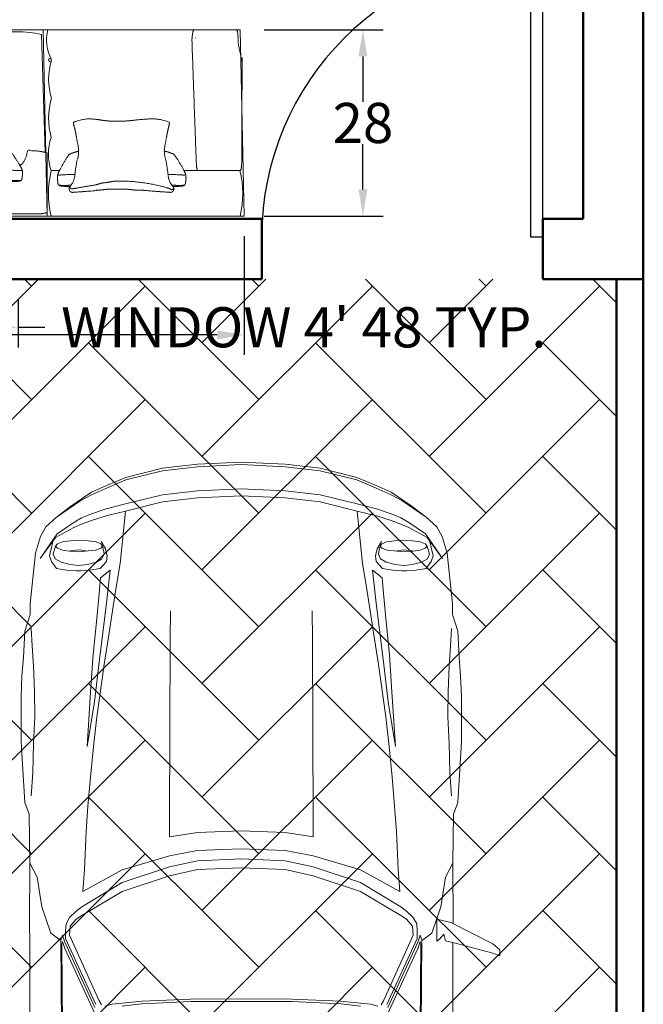
# Model space of a CAD drawing. Units: inches. Extents: x -466983 to 1020, y 324 to 318697.
# Tile 27 of 97: x 899 to 992, y 511 to 658. Entities that reach past the tile are written whole.
import ezdxf

# ---------------------------------------------------------------- set-up
doc = ezdxf.new("R2010")
doc.units = ezdxf.units.IN
doc.header["$MEASUREMENT"] = 0
for name, color, linetype, lineweight in [('A-ANNO-DIMS', 2, 'Continuous', 18), ('A-DOOR', 3, 'Continuous', 25), ('A-EQPM-VEHC', 8, 'Continuous', 18), ('A-FLOR-PATT', 252, 'Continuous', 13), ('A-FURN', 8, 'Continuous', 18), ('A-WALL', 7, 'Continuous', 50)]:
    doc.layers.add(name, color=color, linetype=linetype, lineweight=lineweight)
doc.styles.get("Standard").update_dxf_attribs({"font": 'arial.ttf'})
doc.dimstyles.get("Standard").update_dxf_attribs({"dimtxt": 6, "dimasz": 4, "dimexe": 3, "dimexo": 3, "dimgap": 0.09, "dimtad": 0, "dimtih": 1, "dimtoh": 1, "dimdec": 1, "dimzin": 0, "dimdsep": 46, "dimlunit": 3, "dimtxsty": 'Standard', "dimcen": 0.09, "dimadec": 0, "dimazin": 0, "dimtfac": 1, "dimtdec": 1, "dimtofl": 0, "dimtmove": 0, "dimatfit": 3, "dimfxl": 1, "dimtolj": 1, "dimtzin": 0, "dimarcsym": 0})

# ---------------------------------------------------------------- blocks, each defined once
blk = doc.blocks.new('A$C7AB76BE8')
for p, q in [((1739.9, 1727), (1762, 1752)), ((1762, 1752), (1784, 1752)), ((1784, 1752), (1774.5, 1727)), ((1663.9, 1575), (1739.9, 1727)), ((1774.5, 1727), (1736.1, 1582.3)), ((610.5, 1600.1), (705.5, 1605.7)), ((705.5, 1605.7), (772, 1610.8)), ((772, 1610.8), (847.5, 1613.9)), ((847.5, 1613.9), (920.5, 1613.9)), ((920.5, 1613.9), (1009, 1613.9)), ((1009, 1613.9), (1091.5, 1608.7)), ((1091.5, 1608.7), (1230.5, 1600.1)), ((329, 1562.5), (512.5, 1581.5)), ((512.5, 1581.5), (550.5, 1581.5)), ((550.5, 1581.5), (610.5, 1600.1)), ((601, 1577.2), (664, 1574.1)), ((664, 1574.1), (737, 1569.8)), ((737, 1569.8), (828.5, 1565.5)), ((828.5, 1565.5), (920.5, 1564.6)), ((920.5, 1564.6), (1017.2, 1569)), ((1017.2, 1569), (1123, 1572)), ((1123, 1572), (1206.3, 1578)), ((1230.5, 1600.1), (1271.9, 1585.4)), ((1271.9, 1585.4), (1448.9, 1582.8)), ((1448.9, 1582.8), (1667.8, 1583.2)), ((1499.5, 1556), (1448.9, 1582.8)), ((1651.4, 1524.5), (1663.9, 1575)), ((1736.1, 1582.3), (1729.6, 1556)), ((1736.1, 1582.8), (2641.4, 1581.1)), ((234, 1524.5), (268.5, 1543.5)), ((348.4, 1544.8), (259, 1483.9)), ((268.5, 1543.5), (329, 1562.5)), ((272, 1489.5), (348.4, 1544.8)), ((1607, 1539.2), (1499.5, 1556)), ((1701.9, 1507.2), (1607, 1539.2)), ((1729.6, 1556), (1705, 1549.5)), ((1705, 1549.5), (1723.5, 1534.4)), ((1723.5, 1534.4), (1730.4, 1524.5)), ((199, 1486.5), (234, 1524.5)), ((287.5, 1499), (313, 1505.5)), ((333.3, 1498.6), (303.5, 1489.5)), ((313, 1505.5), (338.5, 1511.5)), ((349.3, 1491.3), (333.3, 1498.6)), ((338.5, 1511.5), (359.6, 1503.8)), ((359.6, 1503.8), (384.7, 1486.5)), ((1730.4, 1524.5), (1651.4, 1524.5)), ((1727.4, 1473.1), (1701.9, 1507.2)), ((139, 1398), (199, 1486.5)), ((161, 1435.6), (199, 1486.5)), ((259, 1483.9), (218, 1423.5)), ((237, 1423.5), (272, 1489.5)), ((284.1, 1436.9), (288.8, 1464.5)), ((288.8, 1464.5), (295.3, 1483)), ((295.3, 1483), (303.5, 1489.5)), ((303.5, 1489.5), (310.9, 1483)), ((310.9, 1483), (317.8, 1464.5)), ((317.8, 1464.5), (322.1, 1439.4)), ((361.8, 1469.2), (349.3, 1491.3)), ((370.4, 1437.3), (361.8, 1469.2)), ((384.7, 1486.5), (391.2, 1448.5)), ((1727.4, 1470.5), (1709.7, 1464.1)), ((1709.7, 1464.1), (1734.3, 1455.8)), ((2913.9, 1461.5), (1727.4, 1470.5)), ((1741.2, 1467.5), (1731.7, 1464.1)), ((1731.7, 1464.1), (1756.8, 1455.8)), ((2189.8, 1462.8), (1741.2, 1467.5)), ((108.8, 1360), (161, 1435.6)), ((218, 1423.5), (202.1, 1395.4)), ((224.5, 1395.4), (237, 1423.5)), ((282.8, 1404), (284.1, 1436.9)), ((321.2, 1436.9), (316.9, 1404)), ((322.1, 1439.4), (324.2, 1404)), ((373.5, 1405.8), (370.4, 1437.3)), ((391.2, 1448.5), (392.5, 1417)), ((1622.1, 1415.3), (1645, 1439)), ((1645, 1439), (1668.7, 1452)), ((1651.4, 1415.3), (1676.9, 1437.3)), ((1668.7, 1452), (1693.7, 1454.1)), ((1676.9, 1437.3), (1709.3, 1439.4)), ((1693.7, 1454.1), (1720.9, 1453.3)), ((1709.3, 1439.4), (1946.3, 1331.9)), ((1720.9, 1453.3), (1959.3, 1344.9)), ((1734.3, 1455.8), (1970.1, 1348.3)), ((1756.8, 1455.8), (1992.5, 1348.3)), ((118.3, 1360), (139, 1398)), ((202.1, 1395.4), (186.5, 1360.4)), ((211.6, 1360.4), (224.5, 1395.4)), ((284.1, 1371.7), (282.8, 1404)), ((316.9, 1404), (322.5, 1372.1)), ((324.2, 1404), (321.2, 1371.7)), ((370.4, 1374.2), (373.5, 1405.8)), ((392.5, 1398), (391.2, 1366)), ((392.5, 1417), (392.5, 1398)), ((1471.8, 1385), (1551.7, 1391.5)), ((1551.7, 1391.5), (1473.1, 1249.5)), ((1519.3, 1249.5), (1607, 1394.5)), ((1551.3, 1249.5), (1637.6, 1394.5)), ((1607, 1394.5), (1622.1, 1415.3)), ((1637.6, 1394.5), (1651.4, 1415.3)), ((85.1, 1306), (108.8, 1360)), ((94.6, 1306), (118.3, 1360)), ((186.5, 1360.4), (169.2, 1306.5)), ((194.3, 1306.5), (211.6, 1360.4)), ((288.8, 1343.6), (284.1, 1371.7)), ((321.2, 1371.7), (318.2, 1345.8)), ((361.8, 1342.3), (370.4, 1374.2)), ((391.2, 1366), (384.7, 1328.1)), ((577.7, 1342.3), (695.1, 1353.5)), ((695.1, 1353.5), (812.5, 1361.7)), ((812.5, 1361.7), (1028, 1376)), ((1028, 1376), (866.5, 1348.8)), ((920.5, 1340.1), (1028, 1352.7)), ((1028, 1352.7), (1138.9, 1363)), ((1138.9, 1363), (1243, 1372.5)), ((1243, 1372.5), (1335, 1379)), ((1335, 1379), (1471.8, 1385)), ((313, 1309.1), (287.5, 1325)), ((295.3, 1326.3), (288.8, 1343.6)), ((303.5, 1320.7), (295.3, 1326.3)), ((311.3, 1326.8), (303.5, 1320.7)), ((303.5, 1320.7), (323.8, 1315.5)), ((318.2, 1345.8), (311.3, 1326.8)), ((333.3, 1313.8), (349.3, 1322)), ((349.3, 1322), (361.8, 1342.3)), ((384.7, 1328.1), (359.6, 1305.6)), ((390.3, 1293.1), (418.8, 1327.6)), ((418.8, 1327.6), (474.9, 1332.4)), ((474.9, 1332.4), (577.7, 1342.3)), ((607, 1318.1), (498.7, 1304.3)), ((711.9, 1330.6), (607, 1318.1)), ((866.5, 1348.8), (711.9, 1330.6)), ((731.4, 1314.7), (920.5, 1340.1)), ((1946.3, 1331.9), (1960.6, 1323.3)), ((55.3, 1236.5), (85.1, 1306)), ((64.8, 1236.5), (94.6, 1306)), ((169.2, 1306.5), (151.5, 1237)), ((177, 1237), (194.3, 1306.5)), ((338.5, 1303), (313, 1309.1)), ((323.8, 1315.5), (333.3, 1313.8)), ((359.6, 1305.6), (338.5, 1303)), ((498.7, 1304.3), (390.3, 1293.1)), ((444.3, 1269.8), (538, 1284.4)), ((538, 1284.4), (639.8, 1299.6)), ((639.8, 1299.6), (731.4, 1314.7)), ((1958.8, 1285.7), (1947.6, 1177.4)), ((1966.2, 1311.6), (1958.8, 1285.7)), ((177, 1237), (366.1, 1256.8)), ((366.1, 1256.8), (444.3, 1269.8)), ((1473.1, 1249.5), (1422.6, 1078.5)), ((1462.3, 1078.5), (1519.3, 1249.5)), ((1494.3, 1078.5), (1551.3, 1249.5)), ((1965.7, 1249.5), (1957.5, 1179.5)), ((22, 1103.5), (55.3, 1236.5)), ((31.5, 1103.5), (64.8, 1236.5)), ((151.5, 1237), (118.3, 1104)), ((143.8, 1104), (177, 1237)), ((1947.6, 1177.4), (1940.7, 1002.1)), ((1957.5, 1179.5), (1948.5, 1002.1)), ((7.8, 977), (22, 1103.5)), ((17.3, 977), (31.5, 1103.5)), ((118.3, 1104), (104.1, 977.5)), ((129.5, 977.5), (143.8, 1104)), ((639.8, 1075.9), (538, 1074.6)), ((1296.5, 1078.1), (639.8, 1075.9)), ((1354.4, 1078.5), (1296.5, 1078.1)), ((1338.8, 977), (1354.4, 1078.5)), ((1422.6, 1078.5), (1403.6, 977)), ((1440.3, 977), (1462.3, 1078.5)), ((1472.3, 977), (1494.3, 1078.5)), ((1940.7, 1002.1), (1939.4, 819)), ((1948.5, 1002.1), (1949.3, 819)), ((0, 819), (7.8, 977)), ((9.1, 819), (17.3, 977)), ((104.1, 977.5), (96.3, 819)), ((121.8, 819), (129.5, 977.5)), ((1332.4, 819), (1338.8, 977)), ((1403.6, 977), (1397.1, 819)), ((1433.8, 819), (1440.3, 977)), ((1465.8, 819), (1472.3, 977)), ((0, 819), (7.8, 661)), ((9.1, 819), (17.3, 661)), ((104.1, 660.6), (96.3, 819)), ((121.8, 819), (129.5, 660.6)), ((1332.4, 819), (1338.8, 661)), ((1403.6, 661), (1397.1, 819)), ((1433.8, 819), (1440.3, 661)), ((1465.8, 819), (1472.3, 661)), ((1940.7, 636), (1939.4, 819)), ((1948.5, 636), (1949.3, 819)), ((7.8, 661), (22, 534.5)), ((17.3, 661), (31.5, 534.5)), ((118.3, 534.1), (104.1, 660.6)), ((129.5, 660.6), (143.8, 534.1)), ((1338.8, 661), (1354.4, 559.5)), ((1422.6, 559.5), (1403.6, 661)), ((1440.3, 661), (1462.3, 559.5)), ((1472.3, 661), (1494.3, 559.5)), ((1947.6, 460.7), (1940.7, 636)), ((1957.5, 458.5), (1948.5, 636)), ((22, 534.5), (55.3, 401.5)), ((31.5, 534.5), (64.8, 401.5)), ((151.5, 401.1), (118.3, 534.1)), ((143.8, 534.1), (177, 401.1)), ((639.8, 562.1), (538, 563.4)), ((1296.5, 560), (639.8, 562.1)), ((1354.4, 559.5), (1296.5, 560)), ((1473.1, 388.6), (1422.6, 559.5)), ((1462.3, 559.5), (1519.3, 388.6)), ((1494.3, 559.5), (1551.3, 388.6)), ((1958.8, 352.3), (1947.6, 460.7)), ((1965.7, 388.6), (1957.5, 458.5)), ((55.3, 401.5), (85.1, 332)), ((64.8, 401.5), (94.6, 332)), ((169.2, 331.6), (151.5, 401.1)), ((177, 401.1), (194.3, 331.6)), ((177, 401.1), (366.1, 381.2)), ((366.1, 381.2), (444.3, 368.3)), ((444.3, 368.3), (538, 353.6)), ((1551.7, 246.5), (1473.1, 388.6)), ((1519.3, 388.6), (1607, 243.5)), ((1551.3, 388.6), (1637.6, 243.5)), ((85.1, 332), (108.8, 278)), ((94.6, 332), (118.3, 278)), ((186.5, 277.6), (169.2, 331.6)), ((194.3, 331.6), (211.6, 277.6)), ((313, 329), (287.5, 313)), ((303.5, 317.3), (323.8, 322.5)), ((338.5, 335), (313, 329)), ((323.8, 322.5), (333.3, 324.2)), ((333.3, 324.2), (349.3, 316)), ((359.6, 332.4), (338.5, 335)), ((384.7, 310), (359.6, 332.4)), ((390.3, 345), (418.8, 310.4)), ((498.7, 333.7), (390.3, 345)), ((607, 319.9), (498.7, 333.7)), ((538, 353.6), (639.8, 338.5)), ((639.8, 338.5), (731.4, 323.4)), ((731.4, 323.4), (920.5, 297.9)), ((1966.2, 326.4), (1958.8, 352.3)), ((288.8, 294.5), (284.1, 266.4)), ((295.3, 311.7), (288.8, 294.5)), ((303.5, 317.3), (295.3, 311.7)), ((311.3, 311.3), (303.5, 317.3)), ((318.2, 292.3), (311.3, 311.3)), ((321.2, 266.4), (318.2, 292.3)), ((349.3, 316), (361.8, 295.7)), ((361.8, 295.7), (370.4, 263.8)), ((391.2, 272), (384.7, 310)), ((418.8, 310.4), (474.9, 305.7)), ((474.9, 305.7), (577.7, 295.7)), ((577.7, 295.7), (695.1, 284.5)), ((711.9, 307.4), (607, 319.9)), ((866.5, 289.3), (711.9, 307.4)), ((1028, 262.1), (866.5, 289.3)), ((920.5, 297.9), (1028, 285.4)), ((1028, 285.4), (1138.9, 275)), ((1709.3, 198.6), (1946.3, 306.1)), ((1720.9, 184.8), (1959.3, 293.2)), ((1734.3, 182.2), (1970.1, 289.7)), ((1756.8, 182.2), (1992.5, 289.7)), ((1946.3, 306.1), (1960.6, 314.7)), ((108.8, 278), (161, 202.5)), ((118.3, 278), (139, 240.1)), ((202.1, 242.6), (186.5, 277.6)), ((211.6, 277.6), (224.5, 242.6)), ((284.1, 266.4), (282.8, 234)), ((316.9, 234), (322.5, 266)), ((324.2, 234), (321.2, 266.4)), ((370.4, 263.8), (373.5, 232.3)), ((392.5, 240.1), (391.2, 272)), ((695.1, 284.5), (812.5, 276.3)), ((812.5, 276.3), (1028, 262.1)), ((1138.9, 275), (1243, 265.5)), ((1243, 265.5), (1335, 259)), ((1335, 259), (1471.8, 253)), ((1471.8, 253), (1551.7, 246.5)), ((139, 240.1), (199, 151.5)), ((218, 214.6), (202.1, 242.6)), ((259, 154.1), (218, 214.6)), ((224.5, 242.6), (237, 214.6)), ((237, 214.6), (272, 148.5)), ((282.8, 234), (284.1, 201.2)), ((321.2, 201.2), (316.9, 234)), ((322.1, 198.6), (324.2, 234)), ((373.5, 232.3), (370.4, 200.8)), ((391.2, 189.5), (392.5, 221.1)), ((392.5, 221.1), (392.5, 240.1)), ((1607, 243.5), (1622.1, 222.8)), ((1622.1, 222.8), (1645, 199)), ((1637.6, 243.5), (1651.4, 222.8)), ((1651.4, 222.8), (1676.9, 200.8)), ((161, 202.5), (199, 151.5)), ((284.1, 201.2), (288.8, 173.6)), ((317.8, 173.6), (322.1, 198.6)), ((370.4, 200.8), (361.8, 168.8)), ((384.7, 151.5), (391.2, 189.5)), ((1645, 199), (1668.7, 186.1)), ((1668.7, 186.1), (1693.7, 183.9)), ((1676.9, 200.8), (1709.3, 198.6)), ((1693.7, 183.9), (1720.9, 184.8)), ((1709.7, 174), (1734.3, 182.2)), ((1731.7, 174), (1756.8, 182.2)), ((199, 151.5), (234, 113.5)), ((348.4, 93.3), (259, 154.1)), ((272, 148.5), (348.4, 93.3)), ((288.8, 173.6), (295.3, 155)), ((295.3, 155), (303.5, 148.5)), ((303.5, 148.5), (310.9, 155)), ((333.3, 139.5), (303.5, 148.5)), ((310.9, 155), (317.8, 173.6)), ((349.3, 146.8), (333.3, 139.5)), ((361.8, 168.8), (349.3, 146.8)), ((359.6, 134.3), (384.7, 151.5)), ((1727.4, 164.9), (1701.9, 130.8)), ((1727.4, 167.5), (1709.7, 174)), ((2913.9, 176.6), (1727.4, 167.5)), ((1741.2, 170.5), (1731.7, 174)), ((2189.8, 175.3), (1741.2, 170.5)), ((234, 113.5), (268.5, 94.6)), ((287.5, 139), (313, 132.5)), ((313, 132.5), (338.5, 126.5)), ((338.5, 126.5), (359.6, 134.3)), ((1701.9, 130.8), (1607, 98.9)), ((268.5, 94.6), (329, 75.6)), ((329, 75.6), (512.5, 56.6)), ((737, 68.2), (828.5, 72.5)), ((828.5, 72.5), (920.5, 73.4)), ((920.5, 73.4), (1017.2, 69.1)), ((1499.5, 82), (1448.9, 55.3)), ((1607, 98.9), (1499.5, 82)), ((512.5, 56.6), (550.5, 56.6)), ((550.5, 56.6), (610.5, 38)), ((601, 60.9), (664, 63.9)), ((610.5, 38), (705.5, 32.4)), ((664, 63.9), (737, 68.2)), ((1017.2, 69.1), (1123, 66.1)), ((1091.5, 29.4), (1230.5, 38)), ((1123, 66.1), (1206.3, 60)), ((1230.5, 38), (1271.9, 52.7)), ((1271.9, 52.7), (1448.9, 55.3)), ((1448.9, 55.3), (1667.8, 54.8)), ((1736.1, 55.3), (1667.8, 54.8)), ((1736.1, 55.3), (2641.4, 57)), ((705.5, 32.4), (772, 27.2)), ((772, 27.2), (847.5, 24.2)), ((847.5, 24.2), (920.5, 24.2)), ((920.5, 24.2), (1009, 24.2)), ((1009, 24.2), (1091.5, 29.4))]:
    blk.add_line(p, q)
blk = doc.blocks.new('*U39')
for p, q in [((0, 0), (0, -6)), ((-40, 0), (-40, -6))]:
    blk.add_line(p, q)
blk.add_lwpolyline([(0, 0), (0, 40), (-1.75, 40), (-1.75, 0)], close=True)
blk.add_arc((0, 0), 40, 90, 180)
blk = doc.blocks.new('Sofa 1.1')
at = {"extrusion": (0, 0, -1)}
for p, q in [((2542.79, 970.73), (2495.8, 970.73)), ((2543.7, 926.21), (2542.79, 970.73)), ((2496.71, 926.21), (2543.7, 926.21))]:
    blk.add_line(p, q, dxfattribs=at)
for p, q in [((2542.79, 970.73), (2495.8, 970.73)), ((2543.7, 926.21), (2542.79, 970.73)), ((2543.7, 926.21), (2542.79, 970.73)), ((2542.79, 970.73), (2589.78, 970.73)), ((2543.7, 926.21), (2542.79, 970.73)), ((2542.79, 970.73), (2589.78, 970.73)), ((2589.78, 970.73), (2590.69, 926.21)), ((2589.78, 970.73), (2590.69, 926.21)), ((2543.25, 941.45), (2542.34, 969.59)), ((2546.68, 937.15), (2544.69, 937.15)), ((2579.67, 937.15), (2576.31, 937.15)), ((2496.71, 926.21), (2543.7, 926.21)), ((2590.69, 926.21), (2543.7, 926.21)), ((2590.69, 926.21), (2543.7, 926.21))]:
    blk.add_line(p, q)
for centre, radius, start, end in [((2552.88, 968.17), 9.33, 164.053, 209.212), ((2536.58, 943.99), 26.24, 77.3212, 102.6788), ((2544.41, 963.51), 0.346, 18.7323, 341.2677), ((2559.56, 958.88), 15.49, 163.0329, 196.9671), ((2561.22, 949.59), 17.15, 163.8796, 195.4668), ((2555.83, 941.08), 11.82, 160.5487, 199.4513), ((2567.38, 931.59), 23.36, 166.2389, 193.3252), ((2567.01, 931.59), 23.36, 346.6748, 13.7611)]:
    blk.add_arc(centre, radius, start, end)
for points in [[(2578.45, 969.97), (2578.58, 970.73), (2578.72, 970.73)], [(2578.72, 970.73), (2583.8, 970.73), (2588.87, 970.73)], [(2588.87, 970.73), (2589.04, 970.73), (2589.19, 969.61)], [(2578.24, 968.38), (2578.26, 968.53), (2578.27, 968.68)], [(2579.36, 937.91), (2579.27, 938.22), (2578.24, 968.38)], [(2578.27, 968.68), (2578.36, 969.67), (2578.45, 969.97)], [(2579.2, 968.79), (2579.17, 968.79), (2579.13, 968.78)], [(2589.19, 969.61), (2589.24, 968.74), (2589.27, 968.15), (2589.29, 967.24), (2590.2, 962.9)], [(2590.2, 964.12), (2590.2, 957.49), (2590.18, 956.59), (2590.15, 956), (2590.1, 938.27)], [(2590.2, 957.55), (2590.2, 953.33), (2590.2, 964.12)], [(2590.2, 962.9), (2590.2, 961.77), (2590.2, 957.55)], [(2549.9, 931.91), (2549.53, 931.87), (2549.07, 932.2), (2548.96, 932.62), (2548.97, 933.11), (2549.58, 933.79), (2550.25, 935.09), (2550.62, 938.67), (2551.39, 941.46), (2550.81, 944.43), (2550.5, 946.25), (2550.18, 947.51), (2549.95, 948.54), (2550.18, 948.74), (2553, 949.52), (2555.58, 949.33), (2557.03, 949.07), (2557.66, 949)], [(2563.32, 949), (2563.95, 949.07), (2566.26, 949.33), (2569.88, 949.52), (2572.7, 948.74), (2572.93, 948.54), (2572.7, 947.51), (2572.38, 946.25), (2572.07, 944.43), (2571.49, 941.46), (2572.26, 938.67), (2572.63, 935.09), (2573.3, 933.79), (2573.91, 933.11), (2573.92, 932.62), (2573.81, 932.2), (2573.35, 931.87), (2572.98, 931.91)], [(2543.7, 941.24), (2543.7, 941.38), (2542.98, 941.5)], [(2543.7, 927.16), (2543.7, 936.33), (2543.7, 941.24)], [(2579.63, 937.15), (2579.49, 937.15), (2579.36, 937.91)], [(2590.1, 938.27), (2589.95, 937.15), (2589.78, 937.15)], [(2537.72, 937.28), (2537.72, 937.31), (2537.71, 937.35)], [(2546.29, 936.24), (2546.29, 936.26), (2546.3, 936.31)], [(2576.7, 936.24), (2576.7, 936.26), (2576.69, 936.31)], [(2589.78, 937.15), (2584.7, 937.15), (2579.63, 937.15)], [(2549.08, 933.18), (2549.41, 932.81), (2549.53, 932.76)], [(2555.24, 933.67), (2556.16, 933.94), (2556.84, 934.13)], [(2556.84, 934.13), (2558.38, 934.31), (2559.47, 934.52)], [(2559.47, 934.52), (2559.81, 934.57), (2560.16, 934.59)], [(2557.01, 932.53), (2556.09, 932.4), (2555.4, 932.42), (2555.46, 932.32), (2552.35, 932.07), (2551.98, 932.06), (2549.9, 931.91)], [(2558.83, 932.68), (2557.83, 932.62), (2557.01, 932.53)], [(2563.97, 932.53), (2563.15, 932.62), (2562.15, 932.68)], [(2572.98, 931.91), (2570.9, 932.06), (2570.53, 932.07), (2567.42, 932.32), (2566.44, 932.42), (2564.9, 932.4), (2563.97, 932.53)], [(2573.45, 932.53), (2573.53, 932.56), (2573.91, 932.76)], [(2534.4, 926.74), (2540.71, 926.75), (2541.57, 926.76), (2542.13, 926.79), (2542.63, 926.85)], [(2542.63, 926.85), (2543.7, 926.99), (2543.7, 927.16)]]:
    blk.add_open_spline(points, degree=2)
for points, knots in [([(2557.66, 949), (2558.97, 948.87), (2559.7, 948.87), (2559.93, 948.87), (2560.16, 948.87)], [50, 50, 50, 51, 51, 52, 52, 52]), ([(2560.16, 948.87), (2560.4, 948.87), (2560.63, 948.87), (2562.02, 948.87), (2563.32, 949)], [0, 0, 0, 1, 1, 2, 2, 2]), ([(2530.74, 942.77), (2532.37, 942.62), (2532.85, 942.49), (2533.78, 942.23), (2534.38, 942.02), (2534.84, 941.81), (2536.18, 940.04), (2536.96, 938.74), (2537.63, 937.62), (2537.71, 937.35)], [0, 0, 0, 1, 1, 2, 3, 4, 5, 5, 6, 6, 6]), ([(2542.98, 941.5), (2542.68, 941.59), (2542.08, 941.68), (2541, 941.82), (2539.13, 941.91), (2538.18, 938.4), (2537.14, 938.42)], [17, 17, 17, 18, 18, 19, 19, 20, 20, 20]), ([(2546.3, 936.31), (2546.37, 936.59), (2546.99, 937.74), (2547.7, 939.08), (2548.92, 940.91), (2549.34, 941.13), (2549.89, 941.35), (2550.73, 941.61), (2550.9, 941.66), (2551.22, 941.71)], [6, 6, 6, 7, 7, 8, 9, 10, 11, 11, 12, 12, 12]), ([(2571.66, 941.73), (2572.06, 941.67), (2572.26, 941.61), (2573.11, 941.35), (2573.65, 941.13), (2574.07, 940.91), (2575.29, 939.08), (2576.01, 937.74), (2576.62, 936.59), (2576.69, 936.31)], [0, 0, 0, 1, 1, 2, 3, 4, 5, 5, 6, 6, 6]), ([(2531.56, 937.33), (2532.56, 937.25), (2533.29, 937.24), (2534.12, 937.23), (2536.48, 937.13), (2537.31, 937.07), (2537.7, 937.13), (2537.72, 937.28)], [0, 0, 0, 1, 1, 2, 3, 4, 5, 5, 5]), ([(2537.71, 937.35), (2537.91, 936.59), (2537.77, 935.63), (2537.71, 935.01), (2537.39, 934.63), (2536.9, 934.55), (2535.74, 934.46), (2533.01, 934.41), (2532.88, 934.41), (2532.75, 934.41)], [6, 6, 6, 7, 8, 9, 10, 11, 12, 12, 13, 13, 13]), ([(2549.15, 933.3), (2547.91, 933.33), (2547.56, 933.36), (2547.03, 933.41), (2546.59, 933.49), (2546.29, 933.89), (2546.24, 934.53), (2546.11, 935.52), (2546.3, 936.31)], [0, 0, 0, 1, 1, 2, 3, 4, 5, 6, 6, 6]), ([(2546.29, 936.24), (2546.31, 936.08), (2546.66, 936.02), (2547.42, 936.08), (2549.57, 936.18), (2550.33, 936.19), (2550.34, 936.19), (2550.35, 936.19)], [0, 0, 0, 1, 2, 3, 4, 4, 5, 5, 5]), ([(2572.53, 936.19), (2572.6, 936.19), (2572.66, 936.19), (2573.42, 936.18), (2575.57, 936.08), (2576.33, 936.02), (2576.68, 936.08), (2576.7, 936.24)], [0, 0, 0, 1, 1, 2, 3, 4, 5, 5, 5]), ([(2576.69, 936.31), (2576.88, 935.52), (2576.75, 934.53), (2576.7, 933.89), (2576.4, 933.49), (2575.96, 933.41), (2575.43, 933.36), (2575.06, 933.33), (2573.73, 933.29)], [6, 6, 6, 7, 8, 9, 10, 11, 11, 12, 12, 12]), ([(2537.44, 934.72), (2536.51, 934.71), (2535.94, 934.71), (2535.22, 934.71), (2533.9, 934.75), (2533.2, 934.77), (2532.43, 934.82)], [0, 0, 0, 1, 1, 2, 2, 3, 3, 3]), ([(2549.4, 933.6), (2548.46, 933.57), (2547.91, 933.57), (2547.39, 933.57), (2546.54, 933.59)], [0, 0, 0, 1, 1, 2, 2, 2]), ([(2549.53, 932.76), (2549.83, 932.75), (2551.44, 933.05), (2553.27, 933.39), (2555.24, 933.67)], [1, 1, 1, 2, 2, 3, 3, 3]), ([(2560.16, 934.59), (2562.65, 934.66), (2565.39, 934.35), (2568.12, 934.04), (2570.25, 933.53), (2572.39, 933.02), (2572.82, 932.83), (2573.24, 932.64), (2573.38, 932.56), (2573.42, 932.54), (2573.45, 932.53)], [6, 6, 6, 7, 7, 8, 8, 9, 9, 10, 10, 11, 11, 11]), ([(2576.45, 933.59), (2575.6, 933.57), (2575.08, 933.57), (2574.5, 933.57), (2573.48, 933.61)], [0, 0, 0, 1, 1, 2, 2, 2]), ([(2562.15, 932.68), (2561.39, 932.69), (2560.62, 932.69), (2560.16, 932.69), (2559.71, 932.69), (2558.93, 932.69), (2558.83, 932.68)], [24, 24, 24, 25, 25, 27, 27, 28, 28, 28])]:
    blk.add_open_spline(points, degree=2, knots=knots)
blk = doc.blocks.new('*D59')
at = {"layer": 'A-ANNO-DIMS', "color": 0, "lineweight": -2, "transparency": 16777216}
for p, q in [((850.44, 615.94), (850.44, 608.74)), ((898.44, 615.94), (898.44, 608.74)), ((854.44, 611.74), (894.44, 611.74)), ((898.44, 611.74), (902.44, 611.74))]:
    blk.add_line(p, q, dxfattribs=at)
at = {"layer": 'A-ANNO-DIMS', "color": 0, "transparency": 16777216}
for points in [[(854.44, 612.4), (854.44, 611.07), (850.44, 611.74)], [(894.44, 612.4), (894.44, 611.07), (898.44, 611.74)]]:
    blk.add_solid(points, dxfattribs=at)
at = {"layer": 'Defpoints', "color": 0, "transparency": 16777216}
for p in [(850.44, 618.94), (898.44, 618.94), (898.44, 611.74)]:
    blk.add_point(p, dxfattribs=at)
at = {"layer": 'A-ANNO-DIMS', "color": 0, "transparency": 16777216, "insert": (941.11, 611.74), "char_height": 6, "attachment_point": 5}
blk.add_mtext("\\A1;WINDOW 4' 48 TYP.", dxfattribs=at)
blk = doc.blocks.new('*D103')
at = {"layer": 'A-ANNO-DIMS', "color": 0, "lineweight": -2, "transparency": 16777216}
for p, q in [((813.91, 625.34), (813.91, 607.6)), ((932.18, 625.34), (932.18, 607.6)), ((817.91, 610.6), (853.76, 610.6)), ((928.18, 610.6), (892.33, 610.6))]:
    blk.add_line(p, q, dxfattribs=at)
at = {"layer": 'A-ANNO-DIMS', "color": 0, "transparency": 16777216}
for points in [[(817.91, 611.26), (817.91, 609.93), (813.91, 610.6)], [(928.18, 611.26), (928.18, 609.93), (932.18, 610.6)]]:
    blk.add_solid(points, dxfattribs=at)
at = {"layer": 'Defpoints', "color": 0, "transparency": 16777216}
for p in [(813.91, 628.34), (932.18, 628.34), (932.18, 610.6)]:
    blk.add_point(p, dxfattribs=at)
at = {"layer": 'A-ANNO-DIMS', "color": 0, "transparency": 16777216, "insert": (873.05, 610.6), "char_height": 6, "attachment_point": 5}
blk.add_mtext('\\A1;SOFA 118', dxfattribs=at)
blk = doc.blocks.new('*D104')
at = {"layer": 'A-ANNO-DIMS', "color": 0, "lineweight": -2, "transparency": 16777216}
for p, q in [((935.18, 656.22), (952.93, 656.22)), ((949.93, 652.22), (949.93, 645.43)), ((949.93, 632.34), (949.93, 639.13)), ((935.18, 628.34), (952.93, 628.34))]:
    blk.add_line(p, q, dxfattribs=at)
at = {"layer": 'A-ANNO-DIMS', "color": 0, "transparency": 16777216}
for points in [[(949.26, 652.22), (950.59, 652.22), (949.93, 656.22)], [(949.26, 632.34), (950.59, 632.34), (949.93, 628.34)]]:
    blk.add_solid(points, dxfattribs=at)
at = {"layer": 'Defpoints', "color": 0, "transparency": 16777216}
for p in [(932.18, 656.22), (949.93, 656.22), (932.18, 628.34)]:
    blk.add_point(p, dxfattribs=at)
at = {"layer": 'A-ANNO-DIMS', "color": 0, "transparency": 16777216, "insert": (949.93, 642.28), "char_height": 6, "attachment_point": 5}
blk.add_mtext('\\A1;28', dxfattribs=at)

msp = doc.modelspace()

# ---------------------------------------------------------------- hatches: boundary and pattern name
at = {"layer": 'A-FLOR-PATT', "transparency": 33554572}
h = msp.add_hatch(dxfattribs=at)
h.set_pattern_fill('ANSI37', color=256, scale=30)
h.set_pattern_definition([(45, (-1212.4137, -290.035), (-2.6516504, 2.6516504), []), (135, (-1212.4137, -290.035), (-2.6516504, -2.6516504), [])])
h.paths.add_polyline_path([(901.81, 1075.94), (900.61, 1075.94), (900.61, 1065.39), (899.39, 1065.39), (898.09, 1065.39), (892.84, 1058.71, -0.258377), (892.19, 1058.35), (879.98, 1058.35, -0.20177), (879.44, 1058.58), (874.08, 1065.39), (872.78, 1065.39), (871.56, 1065.39), (871.56, 1075.94), (813.81, 1075.94), (813.81, 1044.79), (832.39, 1044.79, -0.394795), (848.66, 1028.54), (848.66, 1009.94), (901.81, 1009.94), (901.81, 1015.94), (901.31, 1015.94), (871.31, 1015.94), (871.31, 1017.25), (871.33, 1017.25, -0.401453), (901.31, 1045.94), (901.81, 1045.94)])
edge = h.paths.add_edge_path(flags=16)
edge.add_line((847.77, 1068.95), (847.77, 1073.71))
edge.add_arc((849.23, 1073.71), 1.45, 90, 180, ccw=False)
edge.add_line((849.23, 1075.16), (864.49, 1075.16))
edge.add_arc((864.49, 1073.71), 1.45, 0, 90, ccw=False)
edge.add_line((865.95, 1073.71), (865.95, 1069))
edge.add_arc((832.64, 1068.98), 33.3, -20.6123, 0.0472, ccw=False)
edge.add_ellipse((856.86, 1058.48), major_axis=(0, 10.21), ratio=0.685919, start_angle=100.0088, end_angle=259.9912, ccw=False)
edge.add_arc((881.07, 1068.98), 33.3, 180.0472, 200.6123, ccw=False)
h.paths.add_polyline_path([(853.15, 1066.48), (853.15, 1066.45), (853.15, 1066.45, 0.433107), (852.92, 1066.68), (852.92, 1066.45), (853.15, 1066.45), (853.15, 1066.48), (853.09, 1066.61, 0.697939), (852.7, 1066.45), (852.7, 1066.45), (852.7, 1066.48), (852.92, 1067), (852.92, 1066.68, -0.396254)], flags=0)
h.paths.add_polyline_path([(861.02, 1066.48), (861.02, 1066.45), (861.02, 1066.45, 0.416404), (860.8, 1066.68), (860.8, 1066.45), (861.02, 1066.45), (861.02, 1066.48), (860.97, 1066.61, 0.713344), (860.57, 1066.45), (860.57, 1066.45), (860.57, 1066.48), (860.8, 1067), (860.8, 1066.68, -0.379973)], flags=0)
edge = h.paths.add_edge_path(flags=0)
edge.add_spline(control_points=[(861.13, 1065.79), (861.47, 1065.25), (861.61, 1065.02), (861.98, 1064.37), (862.19, 1063.94), (862.56, 1063.04), (862.72, 1062.56), (862.99, 1061.58), (863.09, 1061.07), (863.25, 1060.03), (863.29, 1059.5), (863.33, 1058.44), (863.32, 1057.91), (863.24, 1056.85), (863.17, 1056.33), (862.97, 1055.31), (862.84, 1054.81), (862.54, 1053.85), (862.36, 1053.39), (861.95, 1052.52), (861.73, 1052.12), (861.23, 1051.36), (860.97, 1051.02), (860.4, 1050.39), (860.11, 1050.12), (859.49, 1049.65), (859.18, 1049.45), (858.53, 1049.13), (858.2, 1049.01), (857.53, 1048.85), (857.2, 1048.81), (856.52, 1048.81), (856.19, 1048.85), (855.52, 1049.01), (855.19, 1049.13), (854.54, 1049.45), (854.23, 1049.64), (853.61, 1050.12), (853.32, 1050.39), (852.75, 1051.01), (852.49, 1051.36), (852, 1052.11), (851.77, 1052.52), (851.36, 1053.39), (851.18, 1053.85), (850.88, 1054.81), (850.75, 1055.31), (850.55, 1056.33), (850.48, 1056.85), (850.4, 1057.9), (850.39, 1058.44), (850.43, 1059.5), (850.47, 1060.03), (850.63, 1061.07), (850.73, 1061.58), (851, 1062.56), (851.16, 1063.04), (851.53, 1063.94), (851.73, 1064.37), (852.11, 1065.02), (852.25, 1065.25), (852.61, 1065.73)], knot_values=[3.915332, 3.915332, 3.915332, 3.915332, 4.013468, 4.013468, 4.175532, 4.175532, 4.337596, 4.337596, 4.49966, 4.49966, 4.661724, 4.661724, 4.823788, 4.823788, 4.985852, 4.985852, 5.147916, 5.147916, 5.30998, 5.30998, 5.472044, 5.472044, 5.634109, 5.634109, 5.796173, 5.796173, 5.958237, 5.958237, 6.120301, 6.120301, 6.282365, 6.282365, 6.444429, 6.444429, 6.606493, 6.606493, 6.768557, 6.768557, 6.930621, 6.930621, 7.092685, 7.092685, 7.254749, 7.254749, 7.416813, 7.416813, 7.578878, 7.578878, 7.740942, 7.740942, 7.903006, 7.903006, 8.06507, 8.06507, 8.227134, 8.227134, 8.389198, 8.389198, 8.551262, 8.551262, 8.65037, 8.65037, 8.65037, 8.65037], degree=3, periodic=0)
edge.add_line((852.64, 1065.79), (861.13, 1065.79))
edge = h.paths.add_edge_path(flags=0)
edge.add_ellipse((856.85, 1057.74), major_axis=(0, 7.79), ratio=0.687861, start_angle=0, end_angle=360)
h.paths.add_polyline_path([(848.86, 1069.39), (848.86, 1073.96, -0.414214), (849.95, 1075.05), (863.77, 1075.05, -0.414214), (864.86, 1073.96), (864.86, 1069.39, -0.388936), (864.52, 1069.03, -0.043561), (849.2, 1069.03, -0.388936)], flags=0)
h.paths.add_polyline_path([(853.1, 1068.11, -1), (852.68, 1068.11, -1)], flags=0)
edge = h.paths.add_edge_path(flags=0)
edge.add_ellipse((856.86, 1057.34), major_axis=(0, 2.21), ratio=0.657164, start_angle=0, end_angle=360)
h.paths.add_polyline_path([(861.04, 1068.11, -1), (860.62, 1068.11, -1)], flags=0)
edge = h.paths.add_edge_path()
edge.add_line((573.95, 1057.34), (573.95, 1075.94))
edge.add_line((573.95, 1075.94), (558.73, 1075.94))
edge.add_line((558.73, 1075.94), (558.73, 1065.39))
edge.add_line((558.73, 1065.39), (557.51, 1065.39))
edge.add_line((557.51, 1065.39), (556.21, 1065.39))
edge.add_line((556.21, 1065.39), (550.95, 1058.71))
edge.add_arc((550.3, 1059.12), 0.765, 270, 327.9483, ccw=False)
edge.add_line((550.3, 1058.35), (538.1, 1058.35))
edge.add_arc((538.1, 1059.12), 0.765, 224.3704, 270, ccw=False)
edge.add_line((537.55, 1058.58), (532.2, 1065.39))
edge.add_line((532.2, 1065.39), (530.9, 1065.39))
edge.add_line((530.9, 1065.39), (529.67, 1065.39))
edge.add_line((529.67, 1065.39), (529.67, 1075.94))
edge.add_line((529.67, 1075.94), (520.81, 1075.94))
edge.add_line((520.81, 1075.94), (520.81, 1045.94))
edge.add_line((520.81, 1045.94), (521.31, 1045.94))
edge.add_arc((521.31, 1015.94), 30, 2.5075, 90, ccw=False)
edge.add_line((551.28, 1017.25), (551.31, 1017.25))
edge.add_line((551.31, 1017.25), (551.31, 1015.94))
edge.add_line((551.31, 1015.94), (520.81, 1015.94))
edge.add_line((520.81, 1015.94), (520.81, 1009.94))
edge.add_line((520.81, 1009.94), (559.19, 1010.4))
edge.add_arc((559.19, 1011.86), 1.45, 180, 270, ccw=False)
edge.add_line((557.74, 1011.86), (557.74, 1016.56))
edge.add_arc((591.04, 1016.59), 33.3, 159.3877, 180.0472, ccw=False)
edge.add_ellipse((566.82, 1027.08), major_axis=(0, 10.21), ratio=0.685919, start_angle=280.0088, end_angle=439.9912, ccw=False)
edge.add_arc((542.61, 1016.59), 33.3, 0.0472, 20.6123, ccw=False)
edge.add_line((575.91, 1016.62), (575.91, 1011.86))
edge.add_arc((574.46, 1011.86), 1.45, -90, 0, ccw=False)
edge.add_line((574.46, 1010.4), (608.81, 1009.94))
edge.add_line((608.81, 1009.94), (608.81, 1041.09))
edge.add_line((608.81, 1041.09), (590.22, 1041.09))
edge.add_arc((590.78, 1057.91), 16.83, 181.9277, 268.1032, ccw=False)
edge = h.paths.add_edge_path()
edge.add_ellipse((494.24, 583.62), major_axis=(0, 10.21), ratio=0.685919, start_angle=280.0088, end_angle=439.9912, ccw=False)
edge.add_arc((470.03, 573.12), 33.3, 0.0472, 20.6123, ccw=False)
edge.add_line((503.33, 573.15), (503.33, 568.39))
edge.add_arc((501.88, 568.39), 1.45, -90, 0, ccw=False)
edge.add_line((501.88, 566.94), (539.81, 566.94))
edge.add_line((539.81, 566.94), (539.81, 572.94))
edge.add_line((539.81, 572.94), (539.31, 572.94))
edge.add_line((539.31, 572.94), (509.31, 572.94))
edge.add_line((509.31, 572.94), (509.31, 574.25))
edge.add_line((509.31, 574.25), (509.33, 574.25))
edge.add_arc((539.31, 572.94), 30, 90, 177.4925, ccw=False)
edge.add_line((539.31, 602.94), (539.81, 602.94))
edge.add_line((539.81, 602.94), (539.81, 626.94))
edge.add_line((539.81, 626.94), (531.77, 626.94))
edge.add_line((531.77, 626.94), (531.77, 616.39))
edge.add_line((531.77, 616.39), (530.55, 616.39))
edge.add_line((530.55, 616.39), (529.25, 616.39))
edge.add_line((529.25, 616.39), (523.71, 609.35))
edge.add_line((523.71, 609.35), (510.78, 609.35))
edge.add_line((510.78, 609.35), (505.24, 616.39))
edge.add_line((505.24, 616.39), (503.94, 616.39))
edge.add_line((503.94, 616.39), (502.72, 616.39))
edge.add_line((502.72, 616.39), (502.72, 626.94))
edge.add_line((502.72, 626.94), (481.7, 626.94))
edge.add_line((481.7, 626.94), (481.7, 611))
edge.add_arc((467.27, 611.47), 14.44, 271.9277, 358.1032, ccw=False)
edge.add_line((467.76, 597.05), (451.81, 597.05))
edge.add_line((451.81, 597.05), (451.81, 584.4))
edge.add_line((451.81, 584.4), (451.81, 566.94))
edge.add_line((451.81, 566.94), (486.61, 566.94))
edge.add_arc((486.61, 568.39), 1.45, 180, 270, ccw=False)
edge.add_line((485.16, 568.39), (485.16, 573.1))
edge.add_arc((518.46, 573.12), 33.3, 159.3877, 180.0472, ccw=False)
h.paths.add_polyline_path([(836.26, 1020.73), (879.89, 1020.73), (879.89, 1039.39), (836.26, 1039.39)], flags=25)
h.paths.add_polyline_path([(549.99, 1036.75), (593.61, 1036.75), (593.61, 1055.41), (549.99, 1055.41)], flags=24)
h.paths.add_polyline_path([(475.12, 595.6), (518.75, 595.6), (518.75, 614.25), (475.12, 614.25)], flags=24)
h = msp.add_hatch(dxfattribs=at)
h.set_pattern_fill('AR-HBONE', color=256, scale=3)
h.set_pattern_definition([(45, (-1212.414, -290.035), (0, 16.97056), [36, -12]), (135, (-1203.928, -281.55), (1e-15, 16.97056), [36, -12])])
h.paths.add_polyline_path([(987.81, 618.94), (813.81, 618.94), (813.81, 368.94), (987.81, 368.94)])

# ---------------------------------------------------------------- linework, layer by layer
at = {"layer": 'A-WALL'}
for p, q in [((991.81, 1084.94), (991.81, 364.94)), ((982.81, 824.94), (982.81, 627.94)), ((934.81, 627.94), (813.81, 627.94)), ((934.81, 627.94), (934.81, 618.94)), ((976.81, 627.94), (976.81, 618.94)), ((982.81, 627.94), (976.81, 627.94)), ((934.81, 618.94), (813.81, 618.94)), ((991.81, 618.94), (976.81, 618.94)), ((987.81, 618.94), (987.81, 364.94))]:
    msp.add_line(p, q, dxfattribs=at)

# ---------------------------------------------------------------- block references
at = {"layer": 'A-DOOR', "xscale": 1.050000000000011, "yscale": 1.050000000000011, "zscale": 1.050000000000011}
msp.add_blockref('*U39', (976.81, 625.24), dxfattribs=at)
at = {"layer": 'A-EQPM-VEHC', "xscale": 0.0413745961844617, "yscale": 0.0413745961844617, "zscale": 0.0413745961844617, "rotation": 270}
msp.add_blockref('A$C7AB76BE8', (897.88, 591.6), dxfattribs=at)
at = {"layer": 'A-FURN', "xscale": 0.6262868215902297, "yscale": 0.6262868215902297, "zscale": 0.6262868215902297}
msp.add_blockref('Sofa 1.1', (-690.33, 48.27), dxfattribs=at)

# ---------------------------------------------------------------- dimensions: what is measured, and where the dimension line sits
at = {"layer": 'A-ANNO-DIMS'}
dim = msp.add_linear_dim(base=(949.93, 656.22), p1=(932.18, 628.34), p2=(932.18, 656.22), angle=90, dimstyle='Standard', override={"dimdec": 0, "dimlfac": 1, "dimrnd": 0, "dimzin": 0, "dimdsep": 46, "dimlunit": 2}, dxfattribs=at)
dim.commit()
dim.dimension.update_dxf_attribs({"geometry": '*D104', "text_midpoint": (949.93, 642.28)})
for base, p1, p2, text, picture, middle in [((898.44, 611.74), (850.44, 618.94), (898.44, 618.94), "WINDOW 4' <> TYP.", '*D59', (941.11, 611.74)), ((932.18, 610.6), (813.91, 628.34), (932.18, 628.34), 'SOFA <>', '*D103', (873.05, 610.6))]:
    dim = msp.add_linear_dim(base=base, p1=p1, p2=p2, text=text, dimstyle='Standard', override={"dimdec": 0, "dimlfac": 1, "dimrnd": 0, "dimzin": 0, "dimdsep": 46, "dimlunit": 2}, dxfattribs=at)
    dim.commit()
    dim.dimension.update_dxf_attribs({"geometry": picture, "text_midpoint": middle})

doc.saveas('drawing.dxf')
